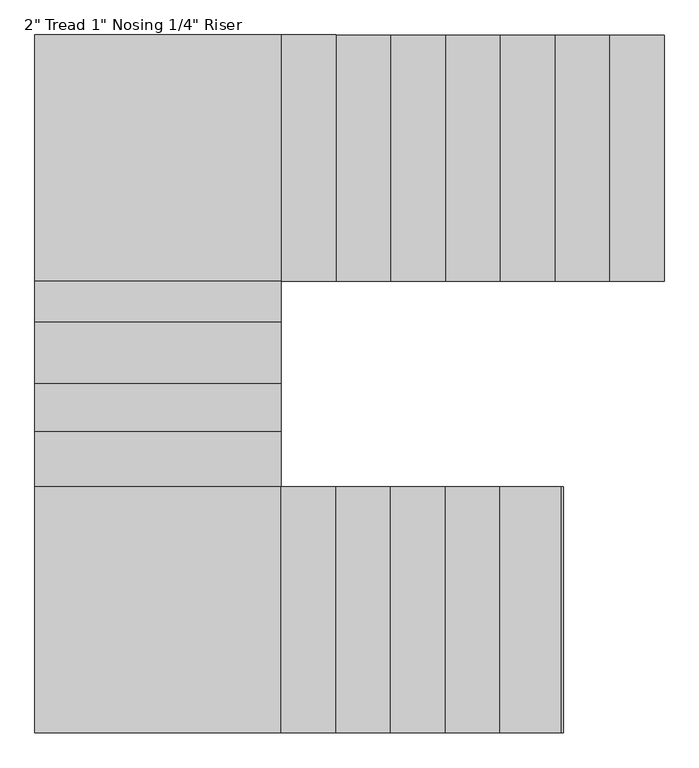
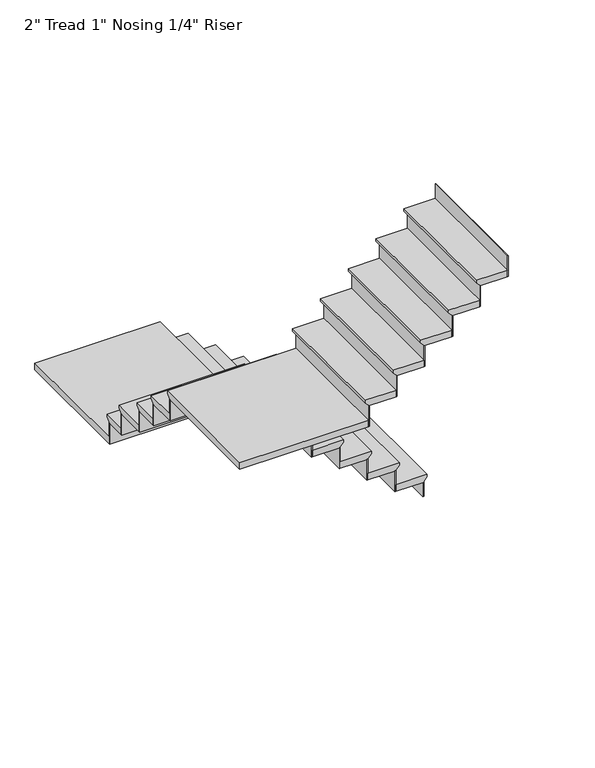
"""IFC4 building model written with IfcOpenShell, lengths in millimetres: stair flight geometry."""

from ifc_helpers import new_model, si_unit, origin, place, context, project, spatial, faceted_brep, source, transform, mapped, element, save


def stair_flight_d806ff93(model_context):
    return source(origin(), model_context, "Body", "Brep", [
        faceted_brep([(-3603.1340247, 922.0319954, 12942.9710526), (-3603.1340247, 922.0319954, 12962.0210526), (-3603.1340247, 7.6319954, 12962.0210526), (-3603.1340247, 7.6319954, 12942.9710526), (-3628.5340247, 922.0319954, 12917.5710526), (-3628.5340247, 7.6319954, 12917.5710526), (-3831.7340247, 922.0319954, 12962.0210526), (-3831.7340247, 7.6319954, 12962.0210526), (-3628.5340247, 7.6319954, 12911.2210526), (-3831.7340247, 7.6319954, 12911.2210526), (-3831.7340247, 922.0319954, 12911.2210526), (-3628.5340247, 922.0319954, 12911.2210526)], [[[0, 1, 2, 3]], [[4, 0, 3, 5]], [[2, 1, 6, 7]], [[8, 9, 10, 11]], [[2, 7, 9, 8, 5, 3]], [[8, 11, 4, 5]], [[6, 1, 0, 4, 11, 10]], [[7, 6, 10, 9]]]),
        faceted_brep([(-3628.5340247, 922.0319954, 12911.2210526), (-3628.5340247, 922.0319954, 12801.6), (-3634.8840247, 922.0319954, 12801.6), (-3634.8840247, 922.0319954, 12911.2210526), (-3628.5340247, 7.6319954, 12911.2210526), (-3634.8840247, 7.6319954, 12911.2210526), (-3634.8840247, 7.6319954, 12801.6), (-3628.5340247, 7.6319954, 12801.6)], [[[0, 1, 2, 3]], [[4, 5, 6, 7]], [[1, 0, 4, 7]], [[2, 1, 7, 6]], [[3, 2, 6, 5]], [[0, 3, 5, 4]]]),
        faceted_brep([(-3831.7340247, 922.0319954, 13071.6421053), (-3831.7340247, 922.0319954, 12911.2210526), (-3838.0840247, 922.0319954, 12911.2210526), (-3838.0840247, 922.0319954, 13071.6421053), (-3831.7340247, 7.6319954, 13071.6421053), (-3838.0840247, 7.6319954, 13071.6421053), (-3838.0840247, 7.6319954, 12911.2210526), (-3831.7340247, 7.6319954, 12911.2210526)], [[[0, 1, 2, 3]], [[4, 5, 6, 7]], [[1, 0, 4, 7]], [[2, 1, 7, 6]], [[3, 2, 6, 5]], [[0, 3, 5, 4]]]),
        faceted_brep([(-3806.3340247, 7.6319954, 13122.4421053), (-3806.3340247, 922.0319954, 13122.4421053), (-4034.9340247, 922.0319954, 13122.4421053), (-4034.9340247, 7.6319954, 13122.4421053), (-3831.7340247, 7.6319954, 13071.6421053), (-4034.9340247, 7.6319954, 13071.6421053), (-4034.9340247, 922.0319954, 13071.6421053), (-3831.7340247, 922.0319954, 13071.6421053), (-3831.7340247, 7.6319954, 13077.9921053), (-3806.3340247, 7.6319954, 13103.3921053), (-3831.7340247, 922.0319954, 13077.9921053), (-3806.3340247, 922.0319954, 13103.3921053)], [[[0, 1, 2, 3]], [[4, 5, 6, 7]], [[0, 3, 5, 4, 8, 9]], [[4, 7, 10, 8]], [[2, 1, 11, 10, 7, 6]], [[3, 2, 6, 5]], [[11, 1, 0, 9]], [[10, 11, 9, 8]]]),
        faceted_brep([(-4034.9340247, 922.0319954, 13232.0631579), (-4034.9340247, 922.0319954, 13071.6421053), (-4041.2840247, 922.0319954, 13071.6421053), (-4041.2840247, 922.0319954, 13232.0631579), (-4034.9340247, 7.6319954, 13232.0631579), (-4041.2840247, 7.6319954, 13232.0631579), (-4041.2840247, 7.6319954, 13071.6421053), (-4034.9340247, 7.6319954, 13071.6421053)], [[[0, 1, 2, 3]], [[4, 5, 6, 7]], [[1, 0, 4, 7]], [[2, 1, 7, 6]], [[3, 2, 6, 5]], [[0, 3, 5, 4]]]),
        faceted_brep([(-4009.5340247, 7.6319954, 13282.8631579), (-4009.5340247, 922.0319954, 13282.8631579), (-4238.1340247, 922.0319954, 13282.8631579), (-4238.1340247, 7.6319954, 13282.8631579), (-4034.9340247, 7.6319954, 13232.0631579), (-4238.1340247, 7.6319954, 13232.0631579), (-4238.1340247, 922.0319954, 13232.0631579), (-4034.9340247, 922.0319954, 13232.0631579), (-4034.9340247, 7.6319954, 13238.4131579), (-4009.5340247, 7.6319954, 13263.8131579), (-4034.9340247, 922.0319954, 13238.4131579), (-4009.5340247, 922.0319954, 13263.8131579)], [[[0, 1, 2, 3]], [[4, 5, 6, 7]], [[0, 3, 5, 4, 8, 9]], [[4, 7, 10, 8]], [[2, 1, 11, 10, 7, 6]], [[3, 2, 6, 5]], [[11, 1, 0, 9]], [[10, 11, 9, 8]]]),
        faceted_brep([(-4238.1340247, 922.0319954, 13392.4842105), (-4238.1340247, 922.0319954, 13232.0631579), (-4244.4840247, 922.0319954, 13232.0631579), (-4244.4840247, 922.0319954, 13392.4842105), (-4238.1340247, 7.6319954, 13392.4842105), (-4244.4840247, 7.6319954, 13392.4842105), (-4244.4840247, 7.6319954, 13232.0631579), (-4238.1340247, 7.6319954, 13232.0631579)], [[[0, 1, 2, 3]], [[4, 5, 6, 7]], [[1, 0, 4, 7]], [[2, 1, 7, 6]], [[3, 2, 6, 5]], [[0, 3, 5, 4]]]),
        faceted_brep([(-4212.7340247, 7.6319954, 13443.2842105), (-4212.7340247, 922.0319954, 13443.2842105), (-4441.3340247, 922.0319954, 13443.2842105), (-4441.3340247, 7.6319954, 13443.2842105), (-4238.1340247, 7.6319954, 13392.4842105), (-4441.3340247, 7.6319954, 13392.4842105), (-4441.3340247, 922.0319954, 13392.4842105), (-4238.1340247, 922.0319954, 13392.4842105), (-4238.1340247, 7.6319954, 13398.8342105), (-4212.7340247, 7.6319954, 13424.2342105), (-4238.1340247, 922.0319954, 13398.8342105), (-4212.7340247, 922.0319954, 13424.2342105)], [[[0, 1, 2, 3]], [[4, 5, 6, 7]], [[0, 3, 5, 4, 8, 9]], [[4, 7, 10, 8]], [[2, 1, 11, 10, 7, 6]], [[3, 2, 6, 5]], [[11, 1, 0, 9]], [[10, 11, 9, 8]]]),
        faceted_brep([(-4441.3340247, 922.0319954, 13552.9052632), (-4441.3340247, 922.0319954, 13392.4842105), (-4447.6840247, 922.0319954, 13392.4842105), (-4447.6840247, 922.0319954, 13552.9052632), (-4441.3340247, 7.6319954, 13552.9052632), (-4447.6840247, 7.6319954, 13552.9052632), (-4447.6840247, 7.6319954, 13392.4842105), (-4441.3340247, 7.6319954, 13392.4842105)], [[[0, 1, 2, 3]], [[4, 5, 6, 7]], [[1, 0, 4, 7]], [[2, 1, 7, 6]], [[3, 2, 6, 5]], [[0, 3, 5, 4]]]),
        faceted_brep([(-4415.9340247, 7.6319954, 13603.7052632), (-4415.9340247, 922.0319954, 13603.7052632), (-4644.5340247, 922.0319954, 13603.7052632), (-4644.5340247, 7.6319954, 13603.7052632), (-4441.3340247, 7.6319954, 13552.9052632), (-4644.5340247, 7.6319954, 13552.9052632), (-4644.5340247, 922.0319954, 13552.9052632), (-4441.3340247, 922.0319954, 13552.9052632), (-4441.3340247, 7.6319954, 13559.2552632), (-4415.9340247, 7.6319954, 13584.6552632), (-4441.3340247, 922.0319954, 13559.2552632), (-4415.9340247, 922.0319954, 13584.6552632)], [[[0, 1, 2, 3]], [[4, 5, 6, 7]], [[0, 3, 5, 4, 8, 9]], [[4, 7, 10, 8]], [[2, 1, 11, 10, 7, 6]], [[3, 2, 6, 5]], [[11, 1, 0, 9]], [[10, 11, 9, 8]]]),
        faceted_brep([(-4644.5340247, 922.0319954, 13713.3263158), (-4644.5340247, 922.0319954, 13552.9052632), (-4650.8840247, 922.0319954, 13552.9052632), (-4650.8840247, 922.0319954, 13713.3263158), (-4644.5340247, 7.6319954, 13713.3263158), (-4650.8840247, 7.6319954, 13713.3263158), (-4650.8840247, 7.6319954, 13552.9052632), (-4644.5340247, 7.6319954, 13552.9052632)], [[[0, 1, 2, 3]], [[4, 5, 6, 7]], [[1, 0, 4, 7]], [[2, 1, 7, 6]], [[3, 2, 6, 5]], [[0, 3, 5, 4]]]),
        faceted_brep([(-4619.1340247, 7.6319954, 13764.1263158), (-4619.1340247, 922.0319954, 13764.1263158), (-4847.7340247, 922.0319954, 13764.1263158), (-4847.7340247, 7.6319954, 13764.1263158), (-4644.5340247, 7.6319954, 13713.3263158), (-4847.7340247, 7.6319954, 13713.3263158), (-4847.7340247, 922.0319954, 13713.3263158), (-4644.5340247, 922.0319954, 13713.3263158), (-4644.5340247, 7.6319954, 13719.6763158), (-4619.1340247, 7.6319954, 13745.0763158), (-4644.5340247, 922.0319954, 13719.6763158), (-4619.1340247, 922.0319954, 13745.0763158)], [[[0, 1, 2, 3]], [[4, 5, 6, 7]], [[0, 3, 5, 4, 8, 9]], [[4, 7, 10, 8]], [[2, 1, 11, 10, 7, 6]], [[3, 2, 6, 5]], [[11, 1, 0, 9]], [[10, 11, 9, 8]]]),
        faceted_brep([(-4847.7340247, 922.0319954, 13873.7473684), (-4847.7340247, 922.0319954, 13713.3263158), (-4854.0840247, 922.0319954, 13713.3263158), (-4854.0840247, 922.0319954, 13873.7473684), (-4847.7340247, 7.6319954, 13873.7473684), (-4854.0840247, 7.6319954, 13873.7473684), (-4854.0840247, 7.6319954, 13713.3263158), (-4847.7340247, 7.6319954, 13713.3263158)], [[[0, 1, 2, 3]], [[4, 5, 6, 7]], [[1, 0, 4, 7]], [[2, 1, 7, 6]], [[3, 2, 6, 5]], [[0, 3, 5, 4]]]),
        faceted_brep([(-4822.3340247, 7.6319954, 13924.5473684), (-4822.3340247, 922.0319954, 13924.5473684), (-5050.9340247, 922.0319954, 13924.5473684), (-5050.9340247, 7.6319954, 13924.5473684), (-4847.7340247, 7.6319954, 13873.7473684), (-5050.9340247, 7.6319954, 13873.7473684), (-5050.9340247, 922.0319954, 13873.7473684), (-4847.7340247, 922.0319954, 13873.7473684), (-4847.7340247, 7.6319954, 13880.0973684), (-4822.3340247, 7.6319954, 13905.4973684), (-4847.7340247, 922.0319954, 13880.0973684), (-4822.3340247, 922.0319954, 13905.4973684)], [[[0, 1, 2, 3]], [[4, 5, 6, 7]], [[0, 3, 5, 4, 8, 9]], [[4, 7, 10, 8]], [[2, 1, 11, 10, 7, 6]], [[3, 2, 6, 5]], [[11, 1, 0, 9]], [[10, 11, 9, 8]]]),
        faceted_brep([(-5050.9340247, 922.0319954, 14034.1684211), (-5050.9340247, 922.0319954, 13873.7473684), (-5057.2840247, 922.0319954, 13873.7473684), (-5057.2840247, 922.0319954, 14034.1684211), (-5050.9340247, 7.6319954, 14034.1684211), (-5057.2840247, 7.6319954, 14034.1684211), (-5057.2840247, 7.6319954, 13873.7473684), (-5050.9340247, 7.6319954, 13873.7473684)], [[[0, 1, 2, 3]], [[4, 5, 6, 7]], [[1, 0, 4, 7]], [[2, 1, 7, 6]], [[3, 2, 6, 5]], [[0, 3, 5, 4]]]),
        faceted_brep([(-5939.9340247, 922.0319954, 14084.9684211), (-5939.9340247, -17.7680046, 14084.9684211), (-5025.5340247, -17.7680046, 14084.9684211), (-5025.5340247, 922.0319954, 14084.9684211), (-5025.5340247, 7.6319954, 14034.1684211), (-5025.5340247, -17.7680046, 14034.1684211), (-5939.9340247, -17.7680046, 14034.1684211), (-5939.9340247, 922.0319954, 14034.1684211), (-5050.9340247, 922.0319954, 14034.1684211), (-5050.9340247, 7.6319954, 14034.1684211), (-5025.5340247, 7.6319954, 14065.9184211), (-5025.5340247, 922.0319954, 14065.9184211), (-5050.9340247, 7.6319954, 14040.5184211), (-5050.9340247, 922.0319954, 14040.5184211)], [[[0, 1, 2, 3]], [[4, 5, 6, 7, 8, 9]], [[3, 2, 5, 4, 10, 11]], [[4, 9, 12, 10]], [[9, 8, 13, 12]], [[0, 3, 11, 13, 8, 7]], [[1, 0, 7, 6]], [[2, 1, 6, 5]], [[13, 11, 10, 12]]]),
        faceted_brep([(-5939.9340247, -17.7680046, 14194.5894737), (-5939.9340247, -17.7680046, 14034.1684211), (-5939.9340247, -24.1180046, 14034.1684211), (-5939.9340247, -24.1180046, 14194.5894737), (-5025.5340247, -17.7680046, 14194.5894737), (-5025.5340247, -24.1180046, 14194.5894737), (-5025.5340247, -24.1180046, 14034.1684211), (-5025.5340247, -17.7680046, 14034.1684211)], [[[0, 1, 2, 3]], [[4, 5, 6, 7]], [[1, 0, 4, 7]], [[2, 1, 7, 6]], [[3, 2, 6, 5]], [[0, 3, 5, 4]]]),
        faceted_brep([(-5025.5340247, 7.6319954, 14245.3894737), (-5939.9340247, 7.6319954, 14245.3894737), (-5939.9340247, -170.1680046, 14245.3894737), (-5025.5340247, -170.1680046, 14245.3894737), (-5025.5340247, -17.7680046, 14194.5894737), (-5025.5340247, -170.1680046, 14194.5894737), (-5939.9340247, -170.1680046, 14194.5894737), (-5939.9340247, -17.7680046, 14194.5894737), (-5025.5340247, -17.7680046, 14200.9394737), (-5025.5340247, 7.6319954, 14226.3394737), (-5939.9340247, -17.7680046, 14200.9394737), (-5939.9340247, 7.6319954, 14226.3394737)], [[[0, 1, 2, 3]], [[4, 5, 6, 7]], [[0, 3, 5, 4, 8, 9]], [[4, 7, 10, 8]], [[2, 1, 11, 10, 7, 6]], [[3, 2, 6, 5]], [[11, 1, 0, 9]], [[10, 11, 9, 8]]]),
        faceted_brep([(-5939.9340247, -170.1680046, 14355.0105263), (-5939.9340247, -170.1680046, 14194.5894737), (-5939.9340247, -176.5180046, 14194.5894737), (-5939.9340247, -176.5180046, 14355.0105263), (-5025.5340247, -170.1680046, 14355.0105263), (-5025.5340247, -176.5180046, 14355.0105263), (-5025.5340247, -176.5180046, 14194.5894737), (-5025.5340247, -170.1680046, 14194.5894737)], [[[0, 1, 2, 3]], [[4, 5, 6, 7]], [[1, 0, 4, 7]], [[2, 1, 7, 6]], [[3, 2, 6, 5]], [[0, 3, 5, 4]]]),
        faceted_brep([(-5025.5340247, -144.7680046, 14405.8105263), (-5939.9340247, -144.7680046, 14405.8105263), (-5939.9340247, -398.7680046, 14405.8105263), (-5025.5340247, -398.7680046, 14405.8105263), (-5025.5340247, -170.1680046, 14355.0105263), (-5025.5340247, -398.7680046, 14355.0105263), (-5939.9340247, -398.7680046, 14355.0105263), (-5939.9340247, -170.1680046, 14355.0105263), (-5025.5340247, -170.1680046, 14361.3605263), (-5025.5340247, -144.7680046, 14386.7605263), (-5939.9340247, -170.1680046, 14361.3605263), (-5939.9340247, -144.7680046, 14386.7605263)], [[[0, 1, 2, 3]], [[4, 5, 6, 7]], [[0, 3, 5, 4, 8, 9]], [[4, 7, 10, 8]], [[2, 1, 11, 10, 7, 6]], [[3, 2, 6, 5]], [[11, 1, 0, 9]], [[10, 11, 9, 8]]]),
        faceted_brep([(-5939.9340247, -398.7680046, 14515.4315789), (-5939.9340247, -398.7680046, 14355.0105263), (-5939.9340247, -405.1180046, 14355.0105263), (-5939.9340247, -405.1180046, 14515.4315789), (-5025.5340247, -398.7680046, 14515.4315789), (-5025.5340247, -405.1180046, 14515.4315789), (-5025.5340247, -405.1180046, 14355.0105263), (-5025.5340247, -398.7680046, 14355.0105263)], [[[0, 1, 2, 3]], [[4, 5, 6, 7]], [[1, 0, 4, 7]], [[2, 1, 7, 6]], [[3, 2, 6, 5]], [[0, 3, 5, 4]]]),
        faceted_brep([(-5025.5340247, -373.3680046, 14566.2315789), (-5939.9340247, -373.3680046, 14566.2315789), (-5939.9340247, -576.5680046, 14566.2315789), (-5025.5340247, -576.5680046, 14566.2315789), (-5025.5340247, -398.7680046, 14515.4315789), (-5025.5340247, -576.5680046, 14515.4315789), (-5939.9340247, -576.5680046, 14515.4315789), (-5939.9340247, -398.7680046, 14515.4315789), (-5025.5340247, -398.7680046, 14521.7815789), (-5025.5340247, -373.3680046, 14547.1815789), (-5939.9340247, -398.7680046, 14521.7815789), (-5939.9340247, -373.3680046, 14547.1815789)], [[[0, 1, 2, 3]], [[4, 5, 6, 7]], [[0, 3, 5, 4, 8, 9]], [[4, 7, 10, 8]], [[2, 1, 11, 10, 7, 6]], [[3, 2, 6, 5]], [[11, 1, 0, 9]], [[10, 11, 9, 8]]]),
        faceted_brep([(-5939.9340247, -576.5680046, 14675.8526316), (-5939.9340247, -576.5680046, 14515.4315789), (-5939.9340247, -582.9180046, 14515.4315789), (-5939.9340247, -582.9180046, 14675.8526316), (-5025.5340247, -576.5680046, 14675.8526316), (-5025.5340247, -582.9180046, 14675.8526316), (-5025.5340247, -582.9180046, 14515.4315789), (-5025.5340247, -576.5680046, 14515.4315789)], [[[0, 1, 2, 3]], [[4, 5, 6, 7]], [[1, 0, 4, 7]], [[2, 1, 7, 6]], [[3, 2, 6, 5]], [[0, 3, 5, 4]]]),
        faceted_brep([(-5025.5340247, -551.1680046, 14726.6526316), (-5939.9340247, -551.1680046, 14726.6526316), (-5939.9340247, -779.7680046, 14726.6526316), (-5025.5340247, -779.7680046, 14726.6526316), (-5025.5340247, -576.5680046, 14675.8526316), (-5025.5340247, -779.7680046, 14675.8526316), (-5939.9340247, -779.7680046, 14675.8526316), (-5939.9340247, -576.5680046, 14675.8526316), (-5025.5340247, -576.5680046, 14682.2026316), (-5025.5340247, -551.1680046, 14707.6026316), (-5939.9340247, -576.5680046, 14682.2026316), (-5939.9340247, -551.1680046, 14707.6026316)], [[[0, 1, 2, 3]], [[4, 5, 6, 7]], [[0, 3, 5, 4, 8, 9]], [[4, 7, 10, 8]], [[2, 1, 11, 10, 7, 6]], [[3, 2, 6, 5]], [[11, 1, 0, 9]], [[10, 11, 9, 8]]]),
        faceted_brep([(-5939.9340247, -779.7680046, 14836.2736842), (-5939.9340247, -779.7680046, 14675.8526316), (-5939.9340247, -786.1180046, 14675.8526316), (-5939.9340247, -786.1180046, 14836.2736842), (-5025.5340247, -779.7680046, 14836.2736842), (-5025.5340247, -786.1180046, 14836.2736842), (-5025.5340247, -786.1180046, 14675.8526316), (-5025.5340247, -779.7680046, 14675.8526316)], [[[0, 1, 2, 3]], [[4, 5, 6, 7]], [[1, 0, 4, 7]], [[2, 1, 7, 6]], [[3, 2, 6, 5]], [[0, 3, 5, 4]]]),
        faceted_brep([(-5939.9340247, -1668.7680046, 14887.0736842), (-5000.1340247, -1668.7680046, 14887.0736842), (-5000.1340247, -754.3680046, 14887.0736842), (-5939.9340247, -754.3680046, 14887.0736842), (-5025.5340247, -754.3680046, 14836.2736842), (-5000.1340247, -754.3680046, 14836.2736842), (-5000.1340247, -1668.7680046, 14836.2736842), (-5939.9340247, -1668.7680046, 14836.2736842), (-5939.9340247, -779.7680046, 14836.2736842), (-5025.5340247, -779.7680046, 14836.2736842), (-5025.5340247, -754.3680046, 14868.0236842), (-5939.9340247, -754.3680046, 14868.0236842), (-5025.5340247, -779.7680046, 14842.6236842), (-5939.9340247, -779.7680046, 14842.6236842)], [[[0, 1, 2, 3]], [[4, 5, 6, 7, 8, 9]], [[3, 2, 5, 4, 10, 11]], [[4, 9, 12, 10]], [[9, 8, 13, 12]], [[0, 3, 11, 13, 8, 7]], [[1, 0, 7, 6]], [[2, 1, 6, 5]], [[13, 11, 10, 12]]]),
        faceted_brep([(-5000.1340247, -1668.7680046, 14996.6947368), (-5000.1340247, -1668.7680046, 14836.2736842), (-4993.7840247, -1668.7680046, 14836.2736842), (-4993.7840247, -1668.7680046, 14996.6947368), (-5000.1340247, -754.3680046, 14996.6947368), (-4993.7840247, -754.3680046, 14996.6947368), (-4993.7840247, -754.3680046, 14836.2736842), (-5000.1340247, -754.3680046, 14836.2736842)], [[[0, 1, 2, 3]], [[4, 5, 6, 7]], [[1, 0, 4, 7]], [[2, 1, 7, 6]], [[3, 2, 6, 5]], [[0, 3, 5, 4]]]),
        faceted_brep([(-5025.5340247, -754.3680046, 15047.4947368), (-5025.5340247, -1668.7680046, 15047.4947368), (-4796.9340247, -1668.7680046, 15047.4947368), (-4796.9340247, -754.3680046, 15047.4947368), (-5000.1340247, -754.3680046, 14996.6947368), (-4796.9340247, -754.3680046, 14996.6947368), (-4796.9340247, -1668.7680046, 14996.6947368), (-5000.1340247, -1668.7680046, 14996.6947368), (-5000.1340247, -754.3680046, 15003.0447368), (-5025.5340247, -754.3680046, 15028.4447368), (-5000.1340247, -1668.7680046, 15003.0447368), (-5025.5340247, -1668.7680046, 15028.4447368)], [[[0, 1, 2, 3]], [[4, 5, 6, 7]], [[0, 3, 5, 4, 8, 9]], [[4, 7, 10, 8]], [[2, 1, 11, 10, 7, 6]], [[3, 2, 6, 5]], [[11, 1, 0, 9]], [[10, 11, 9, 8]]]),
        faceted_brep([(-4796.9340247, -1668.7680046, 15157.1157895), (-4796.9340247, -1668.7680046, 14996.6947368), (-4790.5840247, -1668.7680046, 14996.6947368), (-4790.5840247, -1668.7680046, 15157.1157895), (-4796.9340247, -754.3680046, 15157.1157895), (-4790.5840247, -754.3680046, 15157.1157895), (-4790.5840247, -754.3680046, 14996.6947368), (-4796.9340247, -754.3680046, 14996.6947368)], [[[0, 1, 2, 3]], [[4, 5, 6, 7]], [[1, 0, 4, 7]], [[2, 1, 7, 6]], [[3, 2, 6, 5]], [[0, 3, 5, 4]]]),
        faceted_brep([(-4822.3340247, -754.3680046, 15207.9157895), (-4822.3340247, -1668.7680046, 15207.9157895), (-4593.7340247, -1668.7680046, 15207.9157895), (-4593.7340247, -754.3680046, 15207.9157895), (-4796.9340247, -754.3680046, 15157.1157895), (-4593.7340247, -754.3680046, 15157.1157895), (-4593.7340247, -1668.7680046, 15157.1157895), (-4796.9340247, -1668.7680046, 15157.1157895), (-4796.9340247, -754.3680046, 15163.4657895), (-4822.3340247, -754.3680046, 15188.8657895), (-4796.9340247, -1668.7680046, 15163.4657895), (-4822.3340247, -1668.7680046, 15188.8657895)], [[[0, 1, 2, 3]], [[4, 5, 6, 7]], [[0, 3, 5, 4, 8, 9]], [[4, 7, 10, 8]], [[2, 1, 11, 10, 7, 6]], [[3, 2, 6, 5]], [[11, 1, 0, 9]], [[10, 11, 9, 8]]]),
        faceted_brep([(-4593.7340247, -1668.7680046, 15317.5368421), (-4593.7340247, -1668.7680046, 15157.1157895), (-4587.3840247, -1668.7680046, 15157.1157895), (-4587.3840247, -1668.7680046, 15317.5368421), (-4593.7340247, -754.3680046, 15317.5368421), (-4587.3840247, -754.3680046, 15317.5368421), (-4587.3840247, -754.3680046, 15157.1157895), (-4593.7340247, -754.3680046, 15157.1157895)], [[[0, 1, 2, 3]], [[4, 5, 6, 7]], [[1, 0, 4, 7]], [[2, 1, 7, 6]], [[3, 2, 6, 5]], [[0, 3, 5, 4]]]),
        faceted_brep([(-4619.1340247, -754.3680046, 15368.3368421), (-4619.1340247, -1668.7680046, 15368.3368421), (-4390.5340247, -1668.7680046, 15368.3368421), (-4390.5340247, -754.3680046, 15368.3368421), (-4593.7340247, -754.3680046, 15317.5368421), (-4390.5340247, -754.3680046, 15317.5368421), (-4390.5340247, -1668.7680046, 15317.5368421), (-4593.7340247, -1668.7680046, 15317.5368421), (-4593.7340247, -754.3680046, 15323.8868421), (-4619.1340247, -754.3680046, 15349.2868421), (-4593.7340247, -1668.7680046, 15323.8868421), (-4619.1340247, -1668.7680046, 15349.2868421)], [[[0, 1, 2, 3]], [[4, 5, 6, 7]], [[0, 3, 5, 4, 8, 9]], [[4, 7, 10, 8]], [[2, 1, 11, 10, 7, 6]], [[3, 2, 6, 5]], [[11, 1, 0, 9]], [[10, 11, 9, 8]]]),
        faceted_brep([(-4390.5340247, -1668.7680046, 15477.9578947), (-4390.5340247, -1668.7680046, 15317.5368421), (-4384.1840247, -1668.7680046, 15317.5368421), (-4384.1840247, -1668.7680046, 15477.9578947), (-4390.5340247, -754.3680046, 15477.9578947), (-4384.1840247, -754.3680046, 15477.9578947), (-4384.1840247, -754.3680046, 15317.5368421), (-4390.5340247, -754.3680046, 15317.5368421)], [[[0, 1, 2, 3]], [[4, 5, 6, 7]], [[1, 0, 4, 7]], [[2, 1, 7, 6]], [[3, 2, 6, 5]], [[0, 3, 5, 4]]]),
        faceted_brep([(-4415.9340247, -754.3680046, 15528.7578947), (-4415.9340247, -1668.7680046, 15528.7578947), (-4187.3340247, -1668.7680046, 15528.7578947), (-4187.3340247, -754.3680046, 15528.7578947), (-4390.5340247, -754.3680046, 15477.9578947), (-4187.3340247, -754.3680046, 15477.9578947), (-4187.3340247, -1668.7680046, 15477.9578947), (-4390.5340247, -1668.7680046, 15477.9578947), (-4390.5340247, -754.3680046, 15484.3078947), (-4415.9340247, -754.3680046, 15509.7078947), (-4390.5340247, -1668.7680046, 15484.3078947), (-4415.9340247, -1668.7680046, 15509.7078947)], [[[0, 1, 2, 3]], [[4, 5, 6, 7]], [[0, 3, 5, 4, 8, 9]], [[4, 7, 10, 8]], [[2, 1, 11, 10, 7, 6]], [[3, 2, 6, 5]], [[11, 1, 0, 9]], [[10, 11, 9, 8]]]),
        faceted_brep([(-4187.3340247, -1668.7680046, 15638.3789474), (-4187.3340247, -1668.7680046, 15477.9578947), (-4180.9840247, -1668.7680046, 15477.9578947), (-4180.9840247, -1668.7680046, 15638.3789474), (-4187.3340247, -754.3680046, 15638.3789474), (-4180.9840247, -754.3680046, 15638.3789474), (-4180.9840247, -754.3680046, 15477.9578947), (-4187.3340247, -754.3680046, 15477.9578947)], [[[0, 1, 2, 3]], [[4, 5, 6, 7]], [[1, 0, 4, 7]], [[2, 1, 7, 6]], [[3, 2, 6, 5]], [[0, 3, 5, 4]]]),
        faceted_brep([(-3984.1340247, -1668.7680046, 15798.8), (-3984.1340247, -1668.7680046, 15638.3789474), (-3977.7840247, -1668.7680046, 15638.3789474), (-3977.7840247, -1668.7680046, 15798.8), (-3984.1340247, -754.3680046, 15798.8), (-3977.7840247, -754.3680046, 15798.8), (-3977.7840247, -754.3680046, 15638.3789474), (-3984.1340247, -754.3680046, 15638.3789474)], [[[0, 1, 2, 3]], [[4, 5, 6, 7]], [[1, 0, 4, 7]], [[2, 1, 7, 6]], [[3, 2, 6, 5]], [[0, 3, 5, 4]]]),
        faceted_brep([(-4212.7340247, -754.3680046, 15689.1789474), (-4212.7340247, -1668.7680046, 15689.1789474), (-3984.1340247, -1668.7680046, 15689.1789474), (-3984.1340247, -754.3680046, 15689.1789474), (-4187.3340247, -754.3680046, 15638.3789474), (-3984.1340247, -754.3680046, 15638.3789474), (-3984.1340247, -1668.7680046, 15638.3789474), (-4187.3340247, -1668.7680046, 15638.3789474), (-4187.3340247, -754.3680046, 15644.7289474), (-4212.7340247, -754.3680046, 15670.1289474), (-4187.3340247, -1668.7680046, 15644.7289474), (-4212.7340247, -1668.7680046, 15670.1289474)], [[[0, 1, 2, 3]], [[4, 5, 6, 7]], [[0, 3, 5, 4, 8, 9]], [[4, 7, 10, 8]], [[2, 1, 11, 10, 7, 6]], [[3, 2, 6, 5]], [[11, 1, 0, 9]], [[10, 11, 9, 8]]]),
    ])


if __name__ == "__main__":
    model = new_model("IFC4")
    model_context = context("Model", 3, world=origin())
    ifc_project = project(units=[si_unit("LENGTHUNIT", "METRE", prefix="MILLI")], contexts=[model_context])
    site = spatial("IfcSite", under=ifc_project)
    building = spatial("IfcBuilding", under=site)
    placement = place(None, origin())
    stair_flight_shape = stair_flight_d806ff93(model_context)
    element("IfcStairFlight", 1, ObjectType="2\" Tread 1\" Nosing 1/4\" Riser", at=placement, inside=building, context=model_context, shape_type="MappedRepresentation", body=[
        mapped(stair_flight_shape, transform((0.0, 0.0, 0.0), x_axis=(1.0, 0.0, 0.0), y_axis=(0.0, 1.0, 0.0), z_axis=(0.0, 0.0, 1.0))),
    ])
    save(model, "model.ifc")
